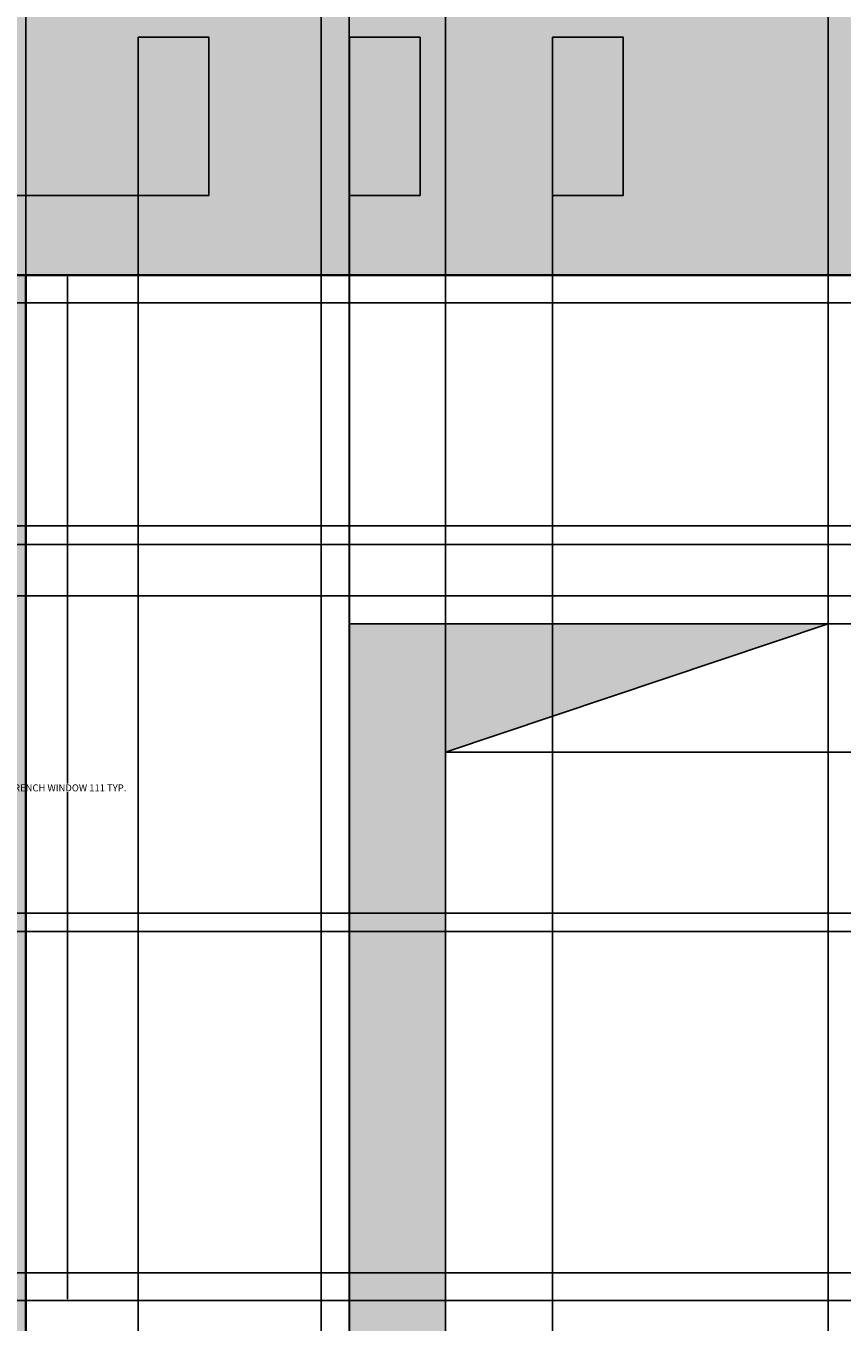
# Model space of a CAD drawing. Units: inches. Extents: x 62 to 566, y 66 to 528.
# Tile 12 of 20: x 284 to 373, y 158 to 298. Entities that reach past the tile are written whole.
import ezdxf

# ---------------------------------------------------------------- set-up
doc = ezdxf.new("R2010")
doc.units = ezdxf.units.IN
doc.header["$MEASUREMENT"] = 0
for name, color, linetype, lineweight in [('A-ANNO-DIMS', 2, 'Continuous', 18), ('A-DOOR', 4, 'Continuous', 25), ('A-ELEV', 7, 'Continuous', 35), ('A-GLAZ', 3, 'Continuous', 25), ('A-WALL-PATT', 8, 'Continuous', 13)]:
    doc.layers.add(name, color=color, linetype=linetype, lineweight=lineweight)
doc.styles.get("Standard").update_dxf_attribs({"font": 'arial.ttf'})
doc.dimstyles.get("Standard").update_dxf_attribs({"dimtxt": 0.75, "dimasz": 0.18, "dimexe": 0.18, "dimexo": 0.0625, "dimgap": 0.09, "dimtad": 0, "dimtih": 1, "dimtoh": 1, "dimdec": 4, "dimzin": 0, "dimdsep": 46, "dimlunit": 4, "dimtxsty": 'Standard', "dimcen": 0.09, "dimadec": 0, "dimazin": 0, "dimtfac": 1, "dimtdec": 4, "dimtofl": 0, "dimtmove": 0, "dimatfit": 3, "dimfxl": 1, "dimtolj": 1, "dimtzin": 0, "dimarcsym": 0})

# ---------------------------------------------------------------- blocks, each defined once
blk = doc.blocks.new('VENT-OPENING')
blk.add_lwpolyline([(0, 17.13), (7.66, 17.13), (7.66, 0), (0, 0)], close=True)
blk = doc.blocks.new('*D5')
at = {"layer": 'A-ANNO-DIMS', "color": 0, "lineweight": -2, "transparency": 16777216}
for p, q in [((272.12, 271.41), (288.9, 271.41)), ((288.72, 271.23), (288.72, 216.36)), ((288.72, 160.53), (288.72, 215.41)), ((272.12, 160.35), (288.9, 160.35))]:
    blk.add_line(p, q, dxfattribs=at)
at = {"layer": 'A-ANNO-DIMS', "color": 0, "transparency": 16777216}
for points in [[(288.69, 271.23), (288.75, 271.23), (288.72, 271.41)], [(288.69, 160.53), (288.75, 160.53), (288.72, 160.35)]]:
    blk.add_solid(points, dxfattribs=at)
at = {"layer": 'Defpoints', "color": 0, "transparency": 16777216}
for p in [(272.06, 271.41), (288.72, 271.41), (272.06, 160.35)]:
    blk.add_point(p, dxfattribs=at)
at = {"layer": 'A-ANNO-DIMS', "color": 0, "transparency": 16777216, "insert": (288.72, 215.88), "char_height": 0.75, "attachment_point": 5}
blk.add_mtext('\\A1;FRENCH WINDOW 111 TYP.', dxfattribs=at)
blk = doc.blocks.new('*D9')
at = {"layer": 'A-ANNO-DIMS', "color": 0, "lineweight": -2, "transparency": 16777216}
for p, q in [((284.2, 271.35), (284.2, 65.94)), ((316.21, 126.31), (316.21, 65.94)), ((284.38, 66.12), (298.92, 66.12)), ((316.03, 66.12), (301.49, 66.12))]:
    blk.add_line(p, q, dxfattribs=at)
at = {"layer": 'A-ANNO-DIMS', "color": 0, "transparency": 16777216}
for points in [[(284.38, 66.15), (284.38, 66.09), (284.2, 66.12)], [(316.03, 66.15), (316.03, 66.09), (316.21, 66.12)]]:
    blk.add_solid(points, dxfattribs=at)
at = {"layer": 'Defpoints', "color": 0, "transparency": 16777216}
for p in [(284.2, 271.41), (316.21, 126.37), (316.21, 66.12)]:
    blk.add_point(p, dxfattribs=at)
at = {"layer": 'A-ANNO-DIMS', "color": 0, "transparency": 16777216, "insert": (300.21, 66.12), "char_height": 0.75, "attachment_point": 5}
blk.add_mtext('\\A1;32.01', dxfattribs=at)
blk = doc.blocks.new('*D10')
at = {"layer": 'A-ANNO-DIMS', "color": 0, "lineweight": -2, "transparency": 16777216}
for p, q in [((396.43, 271.35), (396.43, 65.94)), ((316.21, 126.31), (316.21, 65.94)), ((316.39, 66.12), (354.97, 66.12)), ((396.25, 66.12), (357.67, 66.12))]:
    blk.add_line(p, q, dxfattribs=at)
at = {"layer": 'A-ANNO-DIMS', "color": 0, "transparency": 16777216}
for points in [[(316.39, 66.15), (316.39, 66.09), (316.21, 66.12)], [(396.25, 66.15), (396.25, 66.09), (396.43, 66.12)]]:
    blk.add_solid(points, dxfattribs=at)
at = {"layer": 'Defpoints', "color": 0, "transparency": 16777216}
for p in [(396.43, 271.41), (316.21, 126.37), (396.43, 66.12)]:
    blk.add_point(p, dxfattribs=at)
at = {"layer": 'A-ANNO-DIMS', "color": 0, "transparency": 16777216, "insert": (356.32, 66.12), "char_height": 0.75, "attachment_point": 5}
blk.add_mtext('\\A1;80.22', dxfattribs=at)
blk = doc.blocks.new('*D40')
at = {"layer": 'A-ANNO-DIMS', "color": 0, "lineweight": -2, "transparency": 16777216}
for p, q in [((284.2, 445.04), (284.2, 65.94)), ((316.21, 417.64), (316.21, 65.94)), ((284.38, 66.12), (298.92, 66.12)), ((316.03, 66.12), (301.49, 66.12))]:
    blk.add_line(p, q, dxfattribs=at)
at = {"layer": 'A-ANNO-DIMS', "color": 0, "transparency": 16777216}
for points in [[(284.38, 66.15), (284.38, 66.09), (284.2, 66.12)], [(316.03, 66.15), (316.03, 66.09), (316.21, 66.12)]]:
    blk.add_solid(points, dxfattribs=at)
at = {"layer": 'Defpoints', "color": 0, "transparency": 16777216}
for p in [(284.2, 445.11), (316.21, 417.71), (316.21, 66.12)]:
    blk.add_point(p, dxfattribs=at)
at = {"layer": 'A-ANNO-DIMS', "color": 0, "transparency": 16777216, "insert": (300.21, 66.12), "char_height": 0.75, "attachment_point": 5}
blk.add_mtext('\\A1;32.01', dxfattribs=at)
blk = doc.blocks.new('*D41')
at = {"layer": 'A-ANNO-DIMS', "color": 0, "lineweight": -2, "transparency": 16777216}
for p, q in [((316.21, 417.64), (316.21, 65.94)), ((374.14, 417.64), (374.14, 65.94)), ((316.39, 66.12), (343.82, 66.12)), ((373.96, 66.12), (346.53, 66.12))]:
    blk.add_line(p, q, dxfattribs=at)
at = {"layer": 'A-ANNO-DIMS', "color": 0, "transparency": 16777216}
for points in [[(316.39, 66.15), (316.39, 66.09), (316.21, 66.12)], [(373.96, 66.15), (373.96, 66.09), (374.14, 66.12)]]:
    blk.add_solid(points, dxfattribs=at)
at = {"layer": 'Defpoints', "color": 0, "transparency": 16777216}
for p in [(316.21, 417.71), (374.14, 417.71), (374.14, 66.12)]:
    blk.add_point(p, dxfattribs=at)
at = {"layer": 'A-ANNO-DIMS', "color": 0, "transparency": 16777216, "insert": (345.17, 66.12), "char_height": 0.75, "attachment_point": 5}
blk.add_mtext('\\A1;57.93', dxfattribs=at)
blk = doc.blocks.new('*D61')
at = {"layer": 'A-ANNO-DIMS', "color": 0, "lineweight": -2, "transparency": 16777216}
for p, q in [((316.21, 236.72), (316.21, 527.47)), ((316.39, 527.29), (317.37, 527.29)), ((319.03, 527.29), (318.05, 527.29)), ((319.21, 233.72), (319.21, 527.47))]:
    blk.add_line(p, q, dxfattribs=at)
at = {"layer": 'A-ANNO-DIMS', "color": 0, "transparency": 16777216}
for points in [[(316.39, 527.32), (316.39, 527.26), (316.21, 527.29)], [(319.03, 527.32), (319.03, 527.26), (319.21, 527.29)]]:
    blk.add_solid(points, dxfattribs=at)
at = {"layer": 'Defpoints', "color": 0, "transparency": 16777216}
for p in [(319.21, 527.29), (316.21, 236.66), (319.21, 233.66)]:
    blk.add_point(p, dxfattribs=at)
at = {"layer": 'A-ANNO-DIMS', "color": 0, "transparency": 16777216, "insert": (317.71, 527.29), "char_height": 0.75, "attachment_point": 5}
blk.add_mtext('\\A1;3', dxfattribs=at)
blk = doc.blocks.new('*D62')
at = {"layer": 'A-ANNO-DIMS', "color": 0, "lineweight": -2, "transparency": 16777216}
for p, q in [((319.21, 233.72), (319.21, 527.47)), ((319.39, 527.29), (322.83, 527.29)), ((329.49, 527.29), (326.05, 527.29)), ((329.67, 219.79), (329.67, 527.47))]:
    blk.add_line(p, q, dxfattribs=at)
at = {"layer": 'A-ANNO-DIMS', "color": 0, "transparency": 16777216}
for points in [[(319.39, 527.32), (319.39, 527.26), (319.21, 527.29)], [(329.49, 527.32), (329.49, 527.26), (329.67, 527.29)]]:
    blk.add_solid(points, dxfattribs=at)
at = {"layer": 'Defpoints', "color": 0, "transparency": 16777216}
for p in [(329.67, 527.29), (319.21, 233.66), (329.67, 219.73)]:
    blk.add_point(p, dxfattribs=at)
at = {"layer": 'A-ANNO-DIMS', "color": 0, "transparency": 16777216, "insert": (324.44, 527.29), "char_height": 0.75, "attachment_point": 5}
blk.add_mtext('\\A1;10.456', dxfattribs=at)
blk = doc.blocks.new('*D63')
at = {"layer": 'A-ANNO-DIMS', "color": 0, "lineweight": -2, "transparency": 16777216}
for p, q in [((329.67, 219.79), (329.67, 527.47)), ((329.85, 527.29), (349.03, 527.29)), ((370.96, 527.29), (351.77, 527.29)), ((371.14, 233.72), (371.14, 527.47))]:
    blk.add_line(p, q, dxfattribs=at)
at = {"layer": 'A-ANNO-DIMS', "color": 0, "transparency": 16777216}
for points in [[(329.85, 527.32), (329.85, 527.26), (329.67, 527.29)], [(370.96, 527.32), (370.96, 527.26), (371.14, 527.29)]]:
    blk.add_solid(points, dxfattribs=at)
at = {"layer": 'Defpoints', "color": 0, "transparency": 16777216}
for p in [(371.14, 527.29), (371.14, 233.66), (329.67, 219.73)]:
    blk.add_point(p, dxfattribs=at)
at = {"layer": 'A-ANNO-DIMS', "color": 0, "transparency": 16777216, "insert": (350.4, 527.29), "char_height": 0.75, "attachment_point": 5}
blk.add_mtext('\\A1;41.47', dxfattribs=at)
blk = doc.blocks.new('*D64')
at = {"layer": 'A-ANNO-DIMS', "color": 0, "lineweight": -2, "transparency": 16777216}
for p, q in [((371.14, 233.72), (371.14, 527.47)), ((371.32, 527.29), (372.3, 527.29)), ((373.96, 527.29), (372.97, 527.29)), ((374.14, 236.72), (374.14, 527.47))]:
    blk.add_line(p, q, dxfattribs=at)
at = {"layer": 'A-ANNO-DIMS', "color": 0, "transparency": 16777216}
for points in [[(371.32, 527.32), (371.32, 527.26), (371.14, 527.29)], [(373.96, 527.32), (373.96, 527.26), (374.14, 527.29)]]:
    blk.add_solid(points, dxfattribs=at)
at = {"layer": 'Defpoints', "color": 0, "transparency": 16777216}
for p in [(374.14, 527.29), (374.14, 236.66), (371.14, 233.66)]:
    blk.add_point(p, dxfattribs=at)
at = {"layer": 'A-ANNO-DIMS', "color": 0, "transparency": 16777216, "insert": (372.64, 527.29), "char_height": 0.75, "attachment_point": 5}
blk.add_mtext('\\A1;3', dxfattribs=at)
blk = doc.blocks.new('*D70')
at = {"layer": 'A-ANNO-DIMS', "color": 0, "lineweight": -2, "transparency": 16777216}
for p, q in [((329.73, 219.73), (564.47, 219.73)), ((564.29, 219.55), (564.29, 175.02)), ((564.29, 129.55), (564.29, 174.08)), ((371.2, 129.37), (564.47, 129.37))]:
    blk.add_line(p, q, dxfattribs=at)
at = {"layer": 'A-ANNO-DIMS', "color": 0, "transparency": 16777216}
for points in [[(564.26, 219.55), (564.32, 219.55), (564.29, 219.73)], [(564.26, 129.55), (564.32, 129.55), (564.29, 129.37)]]:
    blk.add_solid(points, dxfattribs=at)
at = {"layer": 'Defpoints', "color": 0, "transparency": 16777216}
for p in [(329.67, 219.73), (564.29, 219.73), (371.14, 129.37)]:
    blk.add_point(p, dxfattribs=at)
at = {"layer": 'A-ANNO-DIMS', "color": 0, "transparency": 16777216, "insert": (564.29, 174.55), "char_height": 0.75, "attachment_point": 5}
blk.add_mtext('\\A1;90.36', dxfattribs=at)
blk = doc.blocks.new('*D71')
at = {"layer": 'A-ANNO-DIMS', "color": 0, "lineweight": -2, "transparency": 16777216}
for p, q in [((371.2, 233.66), (564.47, 233.66)), ((564.29, 233.48), (564.29, 227.17)), ((564.29, 219.91), (564.29, 226.22)), ((329.73, 219.73), (564.47, 219.73))]:
    blk.add_line(p, q, dxfattribs=at)
at = {"layer": 'A-ANNO-DIMS', "color": 0, "transparency": 16777216}
for points in [[(564.26, 233.48), (564.32, 233.48), (564.29, 233.66)], [(564.26, 219.91), (564.32, 219.91), (564.29, 219.73)]]:
    blk.add_solid(points, dxfattribs=at)
at = {"layer": 'Defpoints', "color": 0, "transparency": 16777216}
for p in [(371.14, 233.66), (564.29, 233.66), (329.67, 219.73)]:
    blk.add_point(p, dxfattribs=at)
at = {"layer": 'A-ANNO-DIMS', "color": 0, "transparency": 16777216, "insert": (564.29, 226.7), "char_height": 0.75, "attachment_point": 5}
blk.add_mtext('\\A1;13.93', dxfattribs=at)
blk = doc.blocks.new('*D72')
at = {"layer": 'A-ANNO-DIMS', "color": 0, "lineweight": -2, "transparency": 16777216}
for p, q in [((374.2, 236.66), (564.47, 236.66)), ((564.29, 236.48), (564.29, 235.63)), ((564.29, 233.84), (564.29, 234.69)), ((371.2, 233.66), (564.47, 233.66))]:
    blk.add_line(p, q, dxfattribs=at)
at = {"layer": 'A-ANNO-DIMS', "color": 0, "transparency": 16777216}
for points in [[(564.26, 236.48), (564.32, 236.48), (564.29, 236.66)], [(564.26, 233.84), (564.32, 233.84), (564.29, 233.66)]]:
    blk.add_solid(points, dxfattribs=at)
at = {"layer": 'Defpoints', "color": 0, "transparency": 16777216}
for p in [(374.14, 236.66), (564.29, 236.66), (371.14, 233.66)]:
    blk.add_point(p, dxfattribs=at)
at = {"layer": 'A-ANNO-DIMS', "color": 0, "transparency": 16777216, "insert": (564.29, 235.16), "char_height": 0.75, "attachment_point": 5}
blk.add_mtext('\\A1;3', dxfattribs=at)
blk = doc.blocks.new('*D73')
at = {"layer": 'A-ANNO-DIMS', "color": 0, "lineweight": -2, "transparency": 16777216}
for p, q in [((316.15, 236.66), (63.47, 236.66)), ((63.65, 236.48), (63.65, 181.99)), ((63.65, 126.55), (63.65, 181.04)), ((316.15, 126.37), (63.47, 126.37))]:
    blk.add_line(p, q, dxfattribs=at)
at = {"layer": 'A-ANNO-DIMS', "color": 0, "transparency": 16777216}
for points in [[(63.62, 236.48), (63.68, 236.48), (63.65, 236.66)], [(63.62, 126.55), (63.68, 126.55), (63.65, 126.37)]]:
    blk.add_solid(points, dxfattribs=at)
at = {"layer": 'Defpoints', "color": 0, "transparency": 16777216}
for p in [(63.65, 236.66), (316.21, 236.66), (316.21, 126.37)]:
    blk.add_point(p, dxfattribs=at)
at = {"layer": 'A-ANNO-DIMS', "color": 0, "transparency": 16777216, "insert": (63.65, 181.52), "char_height": 0.75, "attachment_point": 5}
blk.add_mtext('\\A1;110.3', dxfattribs=at)
blk = doc.blocks.new('*D82')
at = {"layer": 'A-ANNO-DIMS', "color": 0, "lineweight": -2, "transparency": 16777216}
for p, q in [((296.38, 279.98), (296.38, 65.94)), ((284.2, 271.35), (284.2, 65.94)), ((284.38, 66.12), (288.68, 66.12)), ((296.2, 66.12), (291.9, 66.12))]:
    blk.add_line(p, q, dxfattribs=at)
at = {"layer": 'A-ANNO-DIMS', "color": 0, "transparency": 16777216}
for points in [[(284.38, 66.15), (284.38, 66.09), (284.2, 66.12)], [(296.2, 66.15), (296.2, 66.09), (296.38, 66.12)]]:
    blk.add_solid(points, dxfattribs=at)
at = {"layer": 'Defpoints', "color": 0, "transparency": 16777216}
for p in [(296.38, 280.04), (284.2, 271.41), (296.38, 66.12)]:
    blk.add_point(p, dxfattribs=at)
at = {"layer": 'A-ANNO-DIMS', "color": 0, "transparency": 16777216, "insert": (290.29, 66.12), "char_height": 0.75, "attachment_point": 5}
blk.add_mtext('\\A1;12.173', dxfattribs=at)
blk = doc.blocks.new('*D83')
at = {"layer": 'A-ANNO-DIMS', "color": 0, "lineweight": -2, "transparency": 16777216}
for p, q in [((296.38, 279.98), (296.38, 65.94)), ((319.25, 279.98), (319.25, 65.94)), ((296.56, 66.12), (306.45, 66.12)), ((319.07, 66.12), (309.18, 66.12))]:
    blk.add_line(p, q, dxfattribs=at)
at = {"layer": 'A-ANNO-DIMS', "color": 0, "transparency": 16777216}
for points in [[(296.56, 66.15), (296.56, 66.09), (296.38, 66.12)], [(319.07, 66.15), (319.07, 66.09), (319.25, 66.12)]]:
    blk.add_solid(points, dxfattribs=at)
at = {"layer": 'Defpoints', "color": 0, "transparency": 16777216}
for p in [(296.38, 280.04), (319.25, 280.04), (319.25, 66.12)]:
    blk.add_point(p, dxfattribs=at)
at = {"layer": 'A-ANNO-DIMS', "color": 0, "transparency": 16777216, "insert": (307.81, 66.12), "char_height": 0.75, "attachment_point": 5}
blk.add_mtext('\\A1;22.88', dxfattribs=at)
blk = doc.blocks.new('*D84')
at = {"layer": 'A-ANNO-DIMS', "color": 0, "lineweight": -2, "transparency": 16777216}
for p, q in [((319.25, 279.98), (319.25, 65.94)), ((341.26, 279.98), (341.26, 65.94)), ((319.43, 66.12), (328.97, 66.12)), ((341.08, 66.12), (331.55, 66.12))]:
    blk.add_line(p, q, dxfattribs=at)
at = {"layer": 'A-ANNO-DIMS', "color": 0, "transparency": 16777216}
for points in [[(319.43, 66.15), (319.43, 66.09), (319.25, 66.12)], [(341.08, 66.15), (341.08, 66.09), (341.26, 66.12)]]:
    blk.add_solid(points, dxfattribs=at)
at = {"layer": 'Defpoints', "color": 0, "transparency": 16777216}
for p in [(319.25, 280.04), (341.26, 280.04), (341.26, 66.12)]:
    blk.add_point(p, dxfattribs=at)
at = {"layer": 'A-ANNO-DIMS', "color": 0, "transparency": 16777216, "insert": (330.26, 66.12), "char_height": 0.75, "attachment_point": 5}
blk.add_mtext('\\A1;22.01', dxfattribs=at)
blk = doc.blocks.new('*D85')
at = {"layer": 'A-ANNO-DIMS', "color": 0, "lineweight": -2, "transparency": 16777216}
for p, q in [((389.29, 281.45), (389.29, 65.94)), ((341.26, 279.98), (341.26, 65.94)), ((341.44, 66.12), (363.91, 66.12)), ((389.11, 66.12), (366.64, 66.12))]:
    blk.add_line(p, q, dxfattribs=at)
at = {"layer": 'A-ANNO-DIMS', "color": 0, "transparency": 16777216}
for points in [[(341.44, 66.15), (341.44, 66.09), (341.26, 66.12)], [(389.11, 66.15), (389.11, 66.09), (389.29, 66.12)]]:
    blk.add_solid(points, dxfattribs=at)
at = {"layer": 'Defpoints', "color": 0, "transparency": 16777216}
for p in [(389.29, 281.51), (341.26, 280.04), (389.29, 66.12)]:
    blk.add_point(p, dxfattribs=at)
at = {"layer": 'A-ANNO-DIMS', "color": 0, "transparency": 16777216, "insert": (365.27, 66.12), "char_height": 0.75, "attachment_point": 5}
blk.add_mtext('\\A1;48.02', dxfattribs=at)
blk = doc.blocks.new('*D98')
at = {"layer": 'A-ANNO-DIMS', "color": 0, "lineweight": -2, "transparency": 16777216}
for p, q in [((296.31, 280.04), (63.47, 280.04)), ((63.65, 279.86), (63.65, 276.2)), ((63.65, 271.59), (63.65, 275.25)), ((284.14, 271.41), (63.47, 271.41))]:
    blk.add_line(p, q, dxfattribs=at)
at = {"layer": 'A-ANNO-DIMS', "color": 0, "transparency": 16777216}
for points in [[(63.62, 279.86), (63.68, 279.86), (63.65, 280.04)], [(63.62, 271.59), (63.68, 271.59), (63.65, 271.41)]]:
    blk.add_solid(points, dxfattribs=at)
at = {"layer": 'Defpoints', "color": 0, "transparency": 16777216}
for p in [(63.65, 280.04), (296.38, 280.04), (284.2, 271.41)]:
    blk.add_point(p, dxfattribs=at)
at = {"layer": 'A-ANNO-DIMS', "color": 0, "transparency": 16777216, "insert": (63.65, 275.73), "char_height": 0.75, "attachment_point": 5}
blk.add_mtext('\\A1;8.63', dxfattribs=at)
blk = doc.blocks.new('*D121')
at = {"layer": 'A-ANNO-DIMS', "color": 0, "lineweight": -2, "transparency": 16777216}
for p, q in [((272.12, 160.35), (564.47, 160.35)), ((564.29, 160.17), (564.29, 158.34)), ((564.29, 155.56), (564.29, 157.39)), ((267.86, 155.38), (564.47, 155.38))]:
    blk.add_line(p, q, dxfattribs=at)
at = {"layer": 'A-ANNO-DIMS', "color": 0, "transparency": 16777216}
for points in [[(564.26, 160.17), (564.32, 160.17), (564.29, 160.35)], [(564.26, 155.56), (564.32, 155.56), (564.29, 155.38)]]:
    blk.add_solid(points, dxfattribs=at)
at = {"layer": 'Defpoints', "color": 0, "transparency": 16777216}
for p in [(272.06, 160.35), (564.29, 160.35), (267.79, 155.38)]:
    blk.add_point(p, dxfattribs=at)
at = {"layer": 'A-ANNO-DIMS', "color": 0, "transparency": 16777216, "insert": (564.29, 157.87), "char_height": 0.75, "attachment_point": 5}
blk.add_mtext('\\A1;4.975', dxfattribs=at)
blk = doc.blocks.new('*D122')
at = {"layer": 'A-ANNO-DIMS', "color": 0, "lineweight": -2, "transparency": 16777216}
for p, q in [((269.12, 163.35), (564.47, 163.35)), ((564.29, 163.17), (564.29, 162.33)), ((272.12, 160.35), (564.47, 160.35)), ((564.29, 160.53), (564.29, 161.38))]:
    blk.add_line(p, q, dxfattribs=at)
at = {"layer": 'A-ANNO-DIMS', "color": 0, "transparency": 16777216}
for points in [[(564.26, 163.17), (564.32, 163.17), (564.29, 163.35)], [(564.26, 160.53), (564.32, 160.53), (564.29, 160.35)]]:
    blk.add_solid(points, dxfattribs=at)
at = {"layer": 'Defpoints', "color": 0, "transparency": 16777216}
for p in [(269.06, 163.35), (564.29, 163.35), (272.06, 160.35)]:
    blk.add_point(p, dxfattribs=at)
at = {"layer": 'A-ANNO-DIMS', "color": 0, "transparency": 16777216, "insert": (564.29, 161.85), "char_height": 0.75, "attachment_point": 5}
blk.add_mtext('\\A1;3', dxfattribs=at)
blk = doc.blocks.new('*D123')
at = {"layer": 'A-ANNO-DIMS', "color": 0, "lineweight": -2, "transparency": 16777216}
for p, q in [((269.12, 200.32), (564.47, 200.32)), ((564.29, 200.14), (564.29, 182.31)), ((564.29, 163.53), (564.29, 181.37)), ((269.12, 163.35), (564.47, 163.35))]:
    blk.add_line(p, q, dxfattribs=at)
at = {"layer": 'A-ANNO-DIMS', "color": 0, "transparency": 16777216}
for points in [[(564.26, 200.14), (564.32, 200.14), (564.29, 200.32)], [(564.26, 163.53), (564.32, 163.53), (564.29, 163.35)]]:
    blk.add_solid(points, dxfattribs=at)
at = {"layer": 'Defpoints', "color": 0, "transparency": 16777216}
for p in [(269.06, 200.32), (564.29, 200.32), (269.06, 163.35)]:
    blk.add_point(p, dxfattribs=at)
at = {"layer": 'A-ANNO-DIMS', "color": 0, "transparency": 16777216, "insert": (564.29, 181.84), "char_height": 0.75, "attachment_point": 5}
blk.add_mtext('\\A1;36.97', dxfattribs=at)
blk = doc.blocks.new('*D124')
at = {"layer": 'A-ANNO-DIMS', "color": 0, "lineweight": -2, "transparency": 16777216}
for p, q in [((269.12, 202.32), (564.47, 202.32)), ((564.29, 202.14), (564.29, 201.79)), ((564.29, 200.5), (564.29, 200.86)), ((269.12, 200.32), (564.47, 200.32))]:
    blk.add_line(p, q, dxfattribs=at)
at = {"layer": 'A-ANNO-DIMS', "color": 0, "transparency": 16777216}
for points in [[(564.26, 202.14), (564.32, 202.14), (564.29, 202.32)], [(564.26, 200.5), (564.32, 200.5), (564.29, 200.32)]]:
    blk.add_solid(points, dxfattribs=at)
at = {"layer": 'Defpoints', "color": 0, "transparency": 16777216}
for p in [(269.06, 202.32), (564.29, 202.32), (269.06, 200.32)]:
    blk.add_point(p, dxfattribs=at)
at = {"layer": 'A-ANNO-DIMS', "color": 0, "transparency": 16777216, "insert": (564.29, 201.32), "char_height": 0.75, "attachment_point": 5}
blk.add_mtext('\\A1;2', dxfattribs=at)
blk = doc.blocks.new('*D125')
at = {"layer": 'A-ANNO-DIMS', "color": 0, "lineweight": -2, "transparency": 16777216}
for p, q in [((269.12, 242.25), (564.47, 242.25)), ((564.29, 242.07), (564.29, 222.76)), ((564.29, 202.5), (564.29, 221.81)), ((269.12, 202.32), (564.47, 202.32))]:
    blk.add_line(p, q, dxfattribs=at)
at = {"layer": 'A-ANNO-DIMS', "color": 0, "transparency": 16777216}
for points in [[(564.26, 242.07), (564.32, 242.07), (564.29, 242.25)], [(564.26, 202.5), (564.32, 202.5), (564.29, 202.32)]]:
    blk.add_solid(points, dxfattribs=at)
at = {"layer": 'Defpoints', "color": 0, "transparency": 16777216}
for p in [(269.06, 242.25), (564.29, 242.25), (269.06, 202.32)]:
    blk.add_point(p, dxfattribs=at)
at = {"layer": 'A-ANNO-DIMS', "color": 0, "transparency": 16777216, "insert": (564.29, 222.29), "char_height": 0.75, "attachment_point": 5}
blk.add_mtext('\\A1;39.93', dxfattribs=at)
blk = doc.blocks.new('*D126')
at = {"layer": 'A-ANNO-DIMS', "color": 0, "lineweight": -2, "transparency": 16777216}
for p, q in [((269.12, 244.25), (564.47, 244.25)), ((564.29, 244.07), (564.29, 243.72)), ((269.12, 242.25), (564.47, 242.25)), ((564.29, 242.43), (564.29, 242.78))]:
    blk.add_line(p, q, dxfattribs=at)
at = {"layer": 'A-ANNO-DIMS', "color": 0, "transparency": 16777216}
for points in [[(564.26, 244.07), (564.32, 244.07), (564.29, 244.25)], [(564.26, 242.43), (564.32, 242.43), (564.29, 242.25)]]:
    blk.add_solid(points, dxfattribs=at)
at = {"layer": 'Defpoints', "color": 0, "transparency": 16777216}
for p in [(269.06, 244.25), (564.29, 244.25), (269.06, 242.25)]:
    blk.add_point(p, dxfattribs=at)
at = {"layer": 'A-ANNO-DIMS', "color": 0, "transparency": 16777216, "insert": (564.29, 243.25), "char_height": 0.75, "attachment_point": 5}
blk.add_mtext('\\A1;2', dxfattribs=at)
blk = doc.blocks.new('*D127')
at = {"layer": 'A-ANNO-DIMS', "color": 0, "lineweight": -2, "transparency": 16777216}
for p, q in [((269.12, 268.41), (564.47, 268.41)), ((564.29, 268.23), (564.29, 256.8)), ((564.29, 244.43), (564.29, 255.86)), ((269.12, 244.25), (564.47, 244.25))]:
    blk.add_line(p, q, dxfattribs=at)
at = {"layer": 'A-ANNO-DIMS', "color": 0, "transparency": 16777216}
for points in [[(564.26, 268.23), (564.32, 268.23), (564.29, 268.41)], [(564.26, 244.43), (564.32, 244.43), (564.29, 244.25)]]:
    blk.add_solid(points, dxfattribs=at)
at = {"layer": 'Defpoints', "color": 0, "transparency": 16777216}
for p in [(269.06, 268.41), (564.29, 268.41), (269.06, 244.25)]:
    blk.add_point(p, dxfattribs=at)
at = {"layer": 'A-ANNO-DIMS', "color": 0, "transparency": 16777216, "insert": (564.29, 256.33), "char_height": 0.75, "attachment_point": 5}
blk.add_mtext('\\A1;24.16', dxfattribs=at)
blk = doc.blocks.new('*D128')
at = {"layer": 'A-ANNO-DIMS', "color": 0, "lineweight": -2, "transparency": 16777216}
for p, q in [((272.12, 271.41), (564.47, 271.41)), ((564.29, 271.23), (564.29, 270.39)), ((269.12, 268.41), (564.47, 268.41)), ((564.29, 268.59), (564.29, 269.44))]:
    blk.add_line(p, q, dxfattribs=at)
at = {"layer": 'A-ANNO-DIMS', "color": 0, "transparency": 16777216}
for points in [[(564.26, 271.23), (564.32, 271.23), (564.29, 271.41)], [(564.26, 268.59), (564.32, 268.59), (564.29, 268.41)]]:
    blk.add_solid(points, dxfattribs=at)
at = {"layer": 'Defpoints', "color": 0, "transparency": 16777216}
for p in [(272.06, 271.41), (564.29, 271.41), (269.06, 268.41)]:
    blk.add_point(p, dxfattribs=at)
at = {"layer": 'A-ANNO-DIMS', "color": 0, "transparency": 16777216, "insert": (564.29, 269.91), "char_height": 0.75, "attachment_point": 5}
blk.add_mtext('\\A1;3', dxfattribs=at)

msp = doc.modelspace()

# ---------------------------------------------------------------- hatches: boundary and pattern name
at = {"layer": 'A-WALL-PATT'}
h = msp.add_hatch(color=256, dxfattribs=at)
h.dxf.hatch_style = 1
h.paths.add_polyline_path([(416.0836, 462.0423), (125.9418, 462.0423), (125.9418, 414.3686), (125.9418, 270.3686), (125.9418, 126.3686), (142.3851, 126.3686), (142.3851, 270.3686), (142.3851, 414.3686), (142.3851, 445.1064), (284.2021, 445.1064), (416.0836, 445.1064)])
h.paths.add_polyline_path([(435.3945, 503.0423), (426.3652, 503.0423), (120.4058, 503.0423), (120.4058, 501.0423), (125.9418, 501.0423), (416.0836, 501.0423), (426.3652, 501.0423), (430.6938, 501.0423), (435.3945, 501.0423)])
h.paths.add_polyline_path([(439.6878, 352.4848), (392.4793, 352.4848), (392.4793, 307.4128), (217.2752, 307.4128), (217.2752, 295.4098), (217.2752, 271.4128), (272.0586, 271.4128), (439.6878, 271.4128)])
h.paths.add_polyline_path([(248.0143, 297.1682), (255.6783, 297.1682), (255.6783, 280.0423), (248.0143, 280.0423)], flags=16)
h.paths.add_polyline_path([(235.4641, 280.0423), (227.8001, 280.0423), (227.8001, 297.1682), (235.4641, 297.1682)], flags=16)
h.paths.add_polyline_path([(270.4427, 297.1682), (278.1067, 297.1682), (278.1067, 280.0423), (270.4427, 280.0423)], flags=16)
h.paths.add_polyline_path([(296.3755, 297.1682), (304.0395, 297.1682), (304.0395, 280.0423), (296.3755, 280.0423)], flags=16)
h.paths.add_polyline_path([(319.2543, 297.1682), (326.9183, 297.1682), (326.9183, 280.0423), (319.2543, 280.0423)], flags=16)
h.paths.add_polyline_path([(341.2622, 297.1682), (348.9262, 297.1682), (348.9262, 280.0423), (341.2622, 280.0423)], flags=16)
h.paths.add_polyline_path([(389.2857, 298.3985), (433.8102, 298.3985), (433.8102, 294.9497), (389.2857, 294.9497)], flags=16)
h.paths.add_polyline_path([(389.2857, 291.6038), (433.8102, 291.6038), (433.8102, 288.155), (389.2857, 288.155)], flags=16)
h.paths.add_polyline_path([(389.2857, 284.9607), (433.8102, 284.9607), (433.8102, 281.5119), (389.2857, 281.5119)], flags=16)
h.paths.add_polyline_path([(403.5849, 311.4736), (403.5849, 317.4388), (433.1636, 317.4388), (433.1636, 311.4736)], flags=16)
h.paths.add_polyline_path([(403.5849, 323.1329), (403.5849, 329.0982), (433.1636, 329.0982), (433.1636, 323.1329)], flags=16)
h.paths.add_polyline_path([(403.5849, 334.5211), (403.5849, 340.4863), (433.1636, 340.4863), (433.1636, 334.5211)], flags=16)
h.paths.add_polyline_path([(272.0586, 160.3545), (217.2752, 160.3545), (217.2752, 129.0504), (217.2752, 126.3686), (272.0586, 126.3686)], flags=17)
h.paths.add_polyline_path([(220.5897, 149.5749), (220.5897, 152.296), (267.7931, 152.296), (267.7931, 149.5749)], flags=16)
h.paths.add_polyline_path([(267.7931, 146.6724), (267.7931, 143.9513), (220.5897, 143.9513), (220.5897, 146.6724)], flags=16)
h.paths.add_polyline_path([(220.5897, 155.3799), (220.5897, 158.101), (267.7931, 158.101), (267.7931, 155.3799)], flags=16)
h.paths.add_polyline_path([(267.7931, 140.686), (267.7931, 137.9649), (220.5897, 137.9649), (220.5897, 140.686)], flags=16)
h.paths.add_polyline_path([(267.7931, 135.516), (267.7931, 132.7949), (220.5897, 132.7949), (220.5897, 135.516)], flags=16)
h = msp.add_hatch(color=256, dxfattribs=at)
h.dxf.hatch_style = 1
h.paths.add_polyline_path([(416.0836, 501.0423), (282.3509, 501.0423), (282.3509, 465.0423), (416.0836, 465.0423)])
h.paths.add_polyline_path([(284.2021, 420.597), (272.0586, 420.597), (272.0586, 309.5388), (272.0586, 307.4128), (284.2021, 307.4128)], flags=17)
h.paths.add_polyline_path([(284.2021, 445.1064), (142.3851, 445.1064), (142.3851, 414.3686), (142.3851, 270.3686), (142.3851, 126.3686), (163.6548, 126.3686), (163.6548, 270.5016), (163.6548, 414.5016), (163.6548, 427.4752), (284.2021, 427.4752)])
h.paths.add_polyline_path([(235.4641, 297.1682), (227.8001, 297.1682), (227.8001, 280.0423), (235.4641, 280.0423)], flags=17)
h.paths.add_polyline_path([(255.6783, 297.1682), (248.0143, 297.1682), (248.0143, 280.0423), (255.6783, 280.0423)], flags=17)
h.paths.add_polyline_path([(278.1067, 297.1682), (270.4427, 297.1682), (270.4427, 280.0423), (278.1067, 280.0423)], flags=17)
h.paths.add_polyline_path([(304.0395, 297.1682), (296.3755, 297.1682), (296.3755, 280.0423), (304.0395, 280.0423)])
h.paths.add_polyline_path([(326.9183, 297.1682), (319.2543, 297.1682), (319.2543, 280.0423), (326.9183, 280.0423)])
h.paths.add_polyline_path([(348.9262, 297.1682), (341.2622, 297.1682), (341.2622, 280.0423), (348.9262, 280.0423)])
h.paths.add_polyline_path([(433.8102, 284.9607), (389.2857, 284.9607), (389.2857, 281.5119), (433.8102, 281.5119)])
h.paths.add_polyline_path([(433.8102, 291.6038), (389.2857, 291.6038), (389.2857, 288.155), (433.8102, 288.155)])
h.paths.add_polyline_path([(433.8102, 298.3985), (389.2857, 298.3985), (389.2857, 294.9497), (433.8102, 294.9497)])
h.paths.add_polyline_path([(433.1636, 317.4388), (403.5849, 317.4388), (403.5849, 311.4736), (433.1636, 311.4736)])
h.paths.add_polyline_path([(433.1636, 329.0982), (403.5849, 329.0982), (403.5849, 323.1329), (433.1636, 323.1329)])
h.paths.add_polyline_path([(433.1636, 340.4863), (403.5849, 340.4863), (403.5849, 334.5211), (433.1636, 334.5211)])
h.paths.add_polyline_path([(284.2021, 271.4128), (272.0586, 271.4128), (272.0586, 160.3545), (272.0586, 126.3686), (284.2021, 126.3686)])
h.paths.add_polyline_path([(267.7931, 158.101), (220.5897, 158.101), (220.5897, 155.3799), (267.7931, 155.3799)], flags=17)
h.paths.add_polyline_path([(267.7931, 152.296), (220.5897, 152.296), (220.5897, 149.5749), (267.7931, 149.5749)], flags=17)
h.paths.add_polyline_path([(267.7931, 146.6724), (220.5897, 146.6724), (220.5897, 143.9513), (267.7931, 143.9513)], flags=17)
h.paths.add_polyline_path([(267.7931, 140.686), (220.5897, 140.686), (220.5897, 137.9649), (267.7931, 137.9649)], flags=17)
h.paths.add_polyline_path([(267.7931, 135.516), (220.5897, 135.516), (220.5897, 132.7949), (267.7931, 132.7949)], flags=17)
h.paths.add_polyline_path([(148.2354, 493.4274), (140.5713, 493.4274), (140.5713, 476.3015), (148.2354, 476.3015)])
h.paths.add_polyline_path([(163.2545, 493.4274), (155.5905, 493.4274), (155.5905, 476.3015), (163.2545, 476.3015)])
h.paths.add_polyline_path([(177.9243, 493.7764), (170.2603, 493.7764), (170.2603, 476.6506), (177.9243, 476.6506)])
h.paths.add_polyline_path([(193.9913, 493.7764), (186.3273, 493.7764), (186.3273, 476.6506), (193.9913, 476.6506)])
h.paths.add_polyline_path([(209.709, 493.7764), (202.045, 493.7764), (202.045, 476.6506), (209.709, 476.6506)])
h = msp.add_hatch(color=256, dxfattribs=at)
h.dxf.hatch_style = 1
h.paths.add_polyline_path([(371.1373, 233.6618), (319.2101, 233.6618), (319.2101, 129.3686), (329.6665, 129.3686), (329.6665, 219.7304)])
h.paths.add_polyline_path([(371.1373, 414.7059), (319.2101, 414.7059), (319.2101, 344.7821), (329.6665, 344.7821), (329.6665, 400.7745)])
h.paths.add_polyline_path([(392.4793, 344.7821), (284.2021, 344.7821), (284.2021, 342.7821), (392.4793, 342.7821)])

# ---------------------------------------------------------------- linework, layer by layer
at = {"layer": 'A-DOOR'}
for p, q in [((371.1373, 233.6618), (329.6665, 219.7304)), ((329.6665, 219.7304), (329.6665, 129.3686))]:
    msp.add_line(p, q, dxfattribs=at)
for points in [[(316.2101, 236.6618), (374.1373, 236.6618), (374.1373, 126.3686), (316.2101, 126.3686)], [(319.2101, 233.6618), (371.1373, 233.6618), (371.1373, 129.3686), (319.2101, 129.3686)]]:
    msp.add_lwpolyline(points, close=True, dxfattribs=at)
at = {"layer": 'A-ELEV'}
for p, q in [((217.2752, 271.4128), (540.0368, 271.4128)), ((284.2021, 126.3686), (284.2021, 271.4128))]:
    msp.add_line(p, q, dxfattribs=at)

# ---------------------------------------------------------------- block references
at = {"layer": 'A-GLAZ'}
for p in [(296.3755, 280.0423), (319.2543, 280.0423), (341.2622, 280.0423)]:
    msp.add_blockref('VENT-OPENING', p, dxfattribs=at)

# ---------------------------------------------------------------- dimensions: what is measured, and where the dimension line sits
at = {"layer": 'A-ANNO-DIMS'}
for base, p1, p2, override, picture, middle in [((319.2101, 527.2923), (316.2101, 236.6618), (319.2101, 233.6618), {"dimdec": 0, "dimlfac": 1, "dimrnd": 0, "dimzin": 0, "dimdsep": 46, "dimlunit": 2}, '*D61', (317.7101, 527.2923)), ((329.6665, 527.2923), (319.2101, 233.6618), (329.6665, 219.7304), {"dimdec": 3, "dimlfac": 1, "dimrnd": 0, "dimzin": 0, "dimdsep": 46, "dimlunit": 2}, '*D62', (324.4383, 527.2923)), ((371.1373, 527.2923), (329.6665, 219.7304), (371.1373, 233.6618), {"dimdec": 2, "dimlfac": 1, "dimrnd": 0, "dimzin": 0, "dimdsep": 46, "dimlunit": 2}, '*D63', (350.4019, 527.2923)), ((374.1373, 527.2923), (371.1373, 233.6618), (374.1373, 236.6618), {"dimdec": 0, "dimlfac": 1, "dimrnd": 0, "dimzin": 0, "dimdsep": 46, "dimlunit": 2}, '*D64', (372.6373, 527.2923)), ((316.2101, 66.1186), (284.2021, 445.1064), (316.2101, 417.7059), {"dimdec": 2, "dimlfac": 1, "dimrnd": 0, "dimzin": 0, "dimdsep": 46, "dimlunit": 2}, '*D40', (300.2061, 66.1186)), ((374.1373, 66.1186), (316.2101, 417.7059), (374.1373, 417.7059), {"dimdec": 2, "dimlfac": 1, "dimrnd": 0, "dimzin": 0, "dimdsep": 46, "dimlunit": 2}, '*D41', (345.1737, 66.1186)), ((389.2857, 66.1186), (341.2622, 280.0423), (389.2857, 281.5119), {"dimdec": 2, "dimlfac": 1, "dimrnd": 0, "dimzin": 0, "dimdsep": 46, "dimlunit": 2}, '*D85', (365.2739, 66.1186)), ((296.3755, 66.1186), (284.2021, 271.4128), (296.3755, 280.0423), {"dimdec": 3, "dimlfac": 1, "dimrnd": 0, "dimzin": 0, "dimdsep": 46, "dimlunit": 2}, '*D82', (290.2888, 66.1186)), ((319.2543, 66.1186), (296.3755, 280.0423), (319.2543, 280.0423), {"dimdec": 2, "dimlfac": 1, "dimrnd": 0, "dimzin": 0, "dimdsep": 46, "dimlunit": 2}, '*D83', (307.8149, 66.1186)), ((341.2622, 66.1186), (319.2543, 280.0423), (341.2622, 280.0423), {"dimdec": 2, "dimlfac": 1, "dimrnd": 0, "dimzin": 0, "dimdsep": 46, "dimlunit": 2}, '*D84', (330.2582, 66.1186)), ((316.2101, 66.1186), (284.2021, 271.4128), (316.2101, 126.3686), {"dimdec": 2, "dimlfac": 1, "dimrnd": 0, "dimzin": 0, "dimdsep": 46, "dimlunit": 2}, '*D9', (300.2061, 66.1186)), ((396.433, 66.1186), (316.2101, 126.3686), (396.433, 271.4128), {"dimdec": 2, "dimlfac": 1, "dimrnd": 0, "dimzin": 0, "dimdsep": 46, "dimlunit": 2}, '*D10', (356.3216, 66.1186))]:
    dim = msp.add_linear_dim(base=base, p1=p1, p2=p2, dimstyle='Standard', override=override, dxfattribs=at)
    dim.commit()
    dim.dimension.update_dxf_attribs({"geometry": picture, "text_midpoint": middle})
for base, p1, p2, override, picture, middle in [((63.6462, 280.0423), (284.2021, 271.4128), (296.3755, 280.0423), {"dimdec": 2, "dimlfac": 1, "dimrnd": 0, "dimzin": 0, "dimdsep": 46, "dimlunit": 2}, '*D98', (63.6462, 275.7276)), ((564.2868, 271.4128), (269.0586, 268.4128), (272.0586, 271.4128), {"dimdec": 0, "dimlfac": 1, "dimrnd": 0, "dimzin": 0, "dimdsep": 46, "dimlunit": 2}, '*D128', (564.2868, 269.9128)), ((564.2868, 268.4128), (269.0586, 244.2507), (269.0586, 268.4128), {"dimdec": 2, "dimlfac": 1, "dimrnd": 0, "dimzin": 0, "dimdsep": 46, "dimlunit": 2}, '*D127', (564.2868, 256.3317)), ((564.2868, 244.2507), (269.0586, 242.2507), (269.0586, 244.2507), {"dimdec": 0, "dimlfac": 1, "dimrnd": 0, "dimzin": 0, "dimdsep": 46, "dimlunit": 2}, '*D126', (564.2868, 243.2507)), ((564.2868, 242.2507), (269.0586, 202.3236), (269.0586, 242.2507), {"dimdec": 2, "dimlfac": 1, "dimrnd": 0, "dimzin": 0, "dimdsep": 46, "dimlunit": 2}, '*D125', (564.2868, 222.2872)), ((63.6462, 236.6618), (316.2101, 126.3686), (316.2101, 236.6618), {"dimdec": 1, "dimlfac": 1, "dimrnd": 0, "dimzin": 0, "dimdsep": 46, "dimlunit": 2}, '*D73', (63.6462, 181.5152)), ((564.2868, 236.6618), (371.1373, 233.6618), (374.1373, 236.6618), {"dimdec": 0, "dimlfac": 1, "dimrnd": 0, "dimzin": 0, "dimdsep": 46, "dimlunit": 2}, '*D72', (564.2868, 235.1618)), ((564.2868, 233.6618), (329.6665, 219.7304), (371.1373, 233.6618), {"dimdec": 2, "dimlfac": 1, "dimrnd": 0, "dimzin": 0, "dimdsep": 46, "dimlunit": 2}, '*D71', (564.2868, 226.6961)), ((564.2868, 219.7304), (371.1373, 129.3686), (329.6665, 219.7304), {"dimdec": 2, "dimlfac": 1, "dimrnd": 0, "dimzin": 0, "dimdsep": 46, "dimlunit": 2}, '*D70', (564.2868, 174.5495)), ((564.2868, 202.3236), (269.0586, 200.3236), (269.0586, 202.3236), {"dimdec": 0, "dimlfac": 1, "dimrnd": 0, "dimzin": 0, "dimdsep": 46, "dimlunit": 2}, '*D124', (564.2868, 201.3236)), ((564.2868, 200.3236), (269.0586, 163.3545), (269.0586, 200.3236), {"dimdec": 2, "dimlfac": 1, "dimrnd": 0, "dimzin": 0, "dimdsep": 46, "dimlunit": 2}, '*D123', (564.2868, 181.8391)), ((564.2868, 163.3545), (272.0586, 160.3545), (269.0586, 163.3545), {"dimdec": 0, "dimlfac": 1, "dimrnd": 0, "dimzin": 0, "dimdsep": 46, "dimlunit": 2}, '*D122', (564.2868, 161.8545)), ((564.2868, 160.3545), (267.7931, 155.3799), (272.0586, 160.3545), {"dimdec": 3, "dimlfac": 1, "dimrnd": 0, "dimzin": 0, "dimdsep": 46, "dimlunit": 2}, '*D121', (564.2868, 157.8672))]:
    dim = msp.add_linear_dim(base=base, p1=p1, p2=p2, angle=90, dimstyle='Standard', override=override, dxfattribs=at)
    dim.commit()
    dim.dimension.update_dxf_attribs({"geometry": picture, "text_midpoint": middle})
dim = msp.add_linear_dim(base=(288.7173, 271.4128), p1=(272.0586, 160.3545), p2=(272.0586, 271.4128), angle=90, text='FRENCH WINDOW <> TYP.', dimstyle='Standard', override={"dimdec": 0, "dimlfac": 1, "dimrnd": 0, "dimzin": 0, "dimdsep": 46, "dimlunit": 2}, dxfattribs=at)
dim.commit()
dim.dimension.update_dxf_attribs({"geometry": '*D5', "text_midpoint": (288.7173, 215.8836)})

doc.saveas('drawing.dxf')
